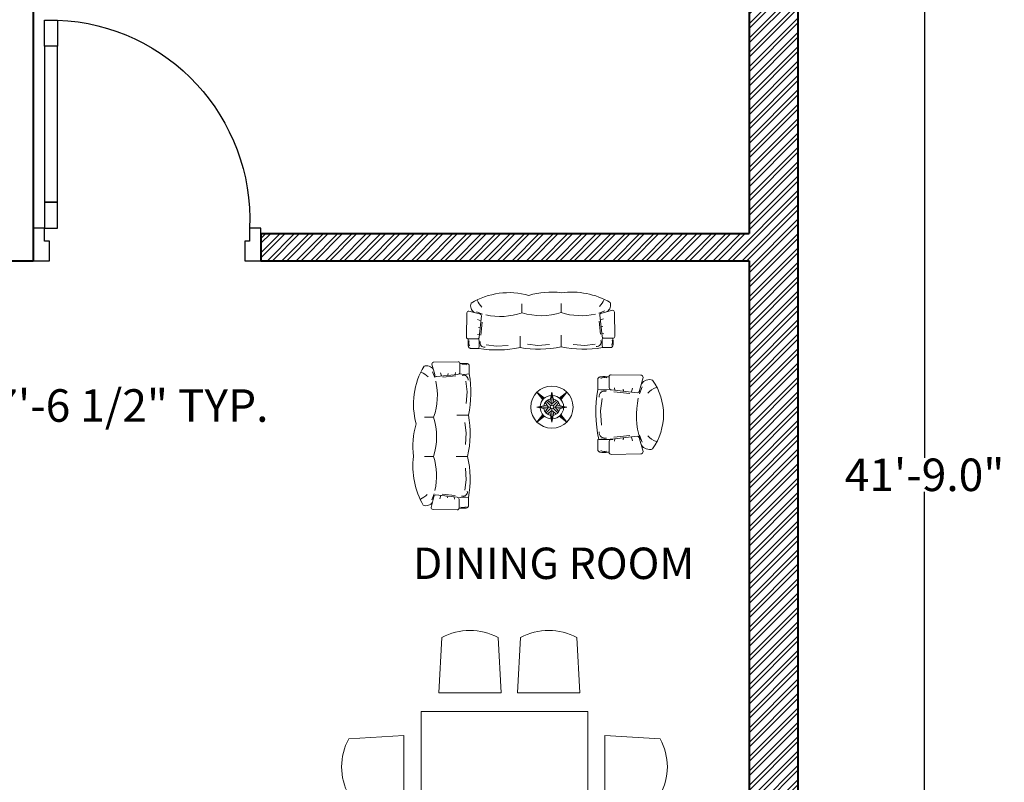
# Model space of a CAD drawing. Units: inches. Extents: x 528 to 2520, y -151 to 1354.
# Tile 21 of 41: x 1279 to 1461, y 1010 to 1151. Entities that reach past the tile are written whole.
import ezdxf

# ---------------------------------------------------------------- set-up
doc = ezdxf.new("R2010")
doc.units = ezdxf.units.IN
doc.header["$MEASUREMENT"] = 0
for name, color, linetype, lineweight in [('A-ANNO-DIMS', 2, 'Continuous', 18), ('A-AREA-IDEN', 7, 'Continuous', 18), ('A-Door', 150, 'Continuous', 25), ('A-FURN', 8, 'Continuous', 18), ('A-WALL-PATT', 6, 'Continuous', 13), ('walls', 7, 'Continuous', 40)]:
    doc.layers.add(name, color=color, linetype=linetype, lineweight=lineweight)
doc.layers.add('NT', color=1, linetype='Continuous')
doc.styles.get("Standard").update_dxf_attribs({"font": 'arial.ttf'})
doc.dimstyles.get("Standard").update_dxf_attribs({"dimtxt": 6, "dimasz": 2, "dimexe": 0.18, "dimexo": 0.0625, "dimgap": 0.09, "dimtad": 0, "dimtih": 1, "dimtoh": 1, "dimdec": 1, "dimzin": 0, "dimdsep": 46, "dimlunit": 3, "dimtxsty": 'Standard', "dimblk": 'ARCHTICK', "dimcen": 0.09, "dimadec": 0, "dimazin": 0, "dimtfac": 1, "dimtdec": 1, "dimtofl": 0, "dimtmove": 0, "dimatfit": 3, "dimfxl": 1, "dimtolj": 1, "dimtzin": 0, "dimarcsym": 0})

# ---------------------------------------------------------------- blocks, each defined once
blk = doc.blocks.new('A$C7DB75F4D')
at = {"layer": 'A-Door'}
for points in [[(625, 740), (625, 660), (665, 660), (665, 740)], [(625, 180), (625, 660), (665, 660), (665, 180)], [(625, 100), (625, 180), (665, 180), (665, 100)], [(35, 100), (35, 60), (50, 60), (50, 50), (50, 0), (0, 0), (0, 100)], [(665, 100), (700, 100), (700, 0), (650, 0), (650, 50), (650, 60), (665, 60)]]:
    blk.add_lwpolyline(points, close=True, dxfattribs=at)
at = {"layer": 'NT'}
blk.add_arc((650, 125), 615.5, 92.3278, 182.3278, dxfattribs=at)
blk = doc.blocks.new('table-20')
at = {"color": 0, "linetype": 'ByBlock'}
for p, q in [((-1.0518, 0.5326), (-1.074, 0.1341)), ((-0.6461, 0.5326), (-0.624, 0.1341)), ((-0.4837, 0.5326), (-0.5058, 0.1341)), ((-0.078, 0.5326), (-0.0558, 0.1341)), ((-0.624, 0.1341), (-1.074, 0.1341)), ((-0.0558, 0.1341), (-0.5058, 0.1341)), ((-1.2, 0), (0, 0)), ((-1.2, -0.8), (-1.2, 0)), ((0, -0.8), (0, 0)), ((-1.7227, -0.1971), (-1.3243, -0.175)), ((-1.3243, -0.625), (-1.3243, -0.175)), ((0.1243, -0.625), (0.1243, -0.175)), ((0.5227, -0.1971), (0.1243, -0.175)), ((-1.7227, -0.6029), (-1.3243, -0.625)), ((0.5227, -0.6029), (0.1243, -0.625)), ((-1.2, -0.8), (0, -0.8)), ((-0.624, -0.9341), (-1.074, -0.9341)), ((-1.0518, -1.3326), (-1.074, -0.9341)), ((-0.6461, -1.3326), (-0.624, -0.9341)), ((-0.4837, -1.3326), (-0.5058, -0.9341)), ((-0.0558, -0.9341), (-0.5058, -0.9341)), ((-0.078, -1.3326), (-0.0558, -0.9341))]:
    blk.add_line(p, q, dxfattribs=at)
for centre, start, end in [((-0.849, 0.1591), 61.48912, 118.51088), ((-0.2808, 0.1591), 61.48912, 118.51088), ((-1.3493, -0.4), 151.48912, 208.51088), ((0.1493, -0.4), 331.48912, 28.51088), ((-0.849, -0.9591), 241.48912, 298.51088), ((-0.2808, -0.9591), 241.48912, 298.51088)]:
    blk.add_arc(centre, 0.425, start, end, dxfattribs=at)
blk = doc.blocks.new('floor')
for p, q in [((-9.5, 11.5), (-18.9, 18.9)), ((-18.9, 18.9), (-10.6, 10.6)), ((-18.9, 18.9), (-11.6, 9.4)), ((0, 18.9), (-2.4, 6.1)), ((2.4, 6.1), (0, 18.9)), ((0, 18.9), (0, 2.1)), ((18.9, 18.9), (9.4, 11.5)), ((18.9, 18.9), (10.6, 10.6)), ((11.5, 9.4), (18.9, 18.9)), ((-6.1, 2.4), (-18.9, 0)), ((-18.9, 0), (-6.1, -2.4)), ((-18.9, 0), (-2.1, 0)), ((-8.7, 5.8), (-4.2, 0)), ((-7.4, 7.4), (-1.5, 1.5)), ((0, 4.2), (-5.8, 8.7)), ((5.8, 8.7), (0, 4.2)), ((7.4, 7.4), (1.5, 1.5)), ((2.1, 0), (18.9, 0)), ((4.2, 0), (8.7, 5.8)), ((18.9, 0), (6.1, 2.4)), ((6.1, -2.4), (18.9, 0)), ((-11.6, -9.5), (-18.9, -18.9)), ((-10.6, -10.6), (-18.9, -18.9)), ((-18.9, -18.9), (-9.5, -11.6)), ((-4.2, 0), (-8.7, -5.8)), ((-1.5, -1.5), (-7.4, -7.4)), ((-5.8, -8.7), (0, -4.2)), ((-2.4, -6.1), (0, -18.9)), ((0, -2.1), (0, -18.9)), ((0, -4.2), (5.8, -8.7)), ((0, -18.9), (2.4, -6.1)), ((1.5, -1.5), (7.4, -7.4)), ((8.7, -5.8), (4.2, 0)), ((9.4, -11.6), (18.9, -18.9)), ((10.6, -10.6), (18.9, -18.9)), ((18.9, -18.9), (11.5, -9.5))]:
    blk.add_line(p, q)
for radius in [26.7, 2.1]:
    blk.add_circle((0, 0), radius)
for radius, start, end in [(14.9, 92.8609, 177.1391), (14.9, 2.8609, 87.1391), (10.5, 98.7017, 171.2983), (10.5, 8.7017, 81.2983), (14.9, 182.8609, 267.1391), (10.5, 188.7017, 261.2983), (14.9, 272.8609, 357.1391), (10.5, 278.7017, 351.2983)]:
    blk.add_arc((0, 0), radius, start, end)
blk = doc.blocks.new('3-s')
for p, q in [((-3104.73, -915.45), (-3104.73, -919.55)), ((-3099.98, -914.27), (-3099.98, -918.75)), ((-3086.85, -913.54), (-3099.1, -913.37)), ((-3087.27, -919.9), (-3085.85, -914.54)), ((-3098.98, -919.75), (-3088.27, -920.9)), ((-3091.42, -921.25), (-3098, -920.58)), ((-3097.59, -919.77), (-3097.73, -918.83)), ((-3093.97, -920.17), (-3094.1, -919.37)), ((-3090.75, -920.58), (-3090.21, -918.96)), ((-3086.18, -918.42), (-3087.39, -921.38)), ((-3102.96, -923.27), (-3103.63, -928.52)), ((-3103.63, -928.52), (-3103.23, -934.44)), ((-3104.33, -940.39), (-3098.51, -940.39)), ((-3087.08, -940.39), (-3082.49, -940.39)), ((-3103.63, -952.27), (-3103.23, -946.35)), ((-3102.96, -957.52), (-3103.63, -952.27)), ((-3087.15, -960.23), (-3082.56, -960.23)), ((-3104.73, -961.23), (-3098.92, -961.23)), ((-3104.04, -973.11), (-3103.63, -967.19)), ((-3103.37, -978.36), (-3104.04, -973.11)), ((-3091.82, -980.37), (-3098.4, -981.05)), ((-3086.59, -983.2), (-3087.79, -980.24)), ((-3105.14, -986.18), (-3105.14, -982.07)), ((-3098, -981.85), (-3098.13, -982.8)), ((-3094.37, -981.45), (-3094.51, -982.26)), ((-3091.15, -981.05), (-3090.61, -982.66))]:
    blk.add_line(p, q)
for points in [[(-3099.98, -914.27), (-3100.65, -914.23), (-3101.21, -914.21), (-3101.68, -914.19), (-3102.07, -914.18), (-3102.4, -914.18), (-3102.68, -914.19), (-3102.91, -914.21), (-3103.11, -914.22), (-3103.29, -914.24), (-3103.46, -914.26), (-3103.62, -914.29), (-3103.76, -914.33), (-3103.89, -914.36), (-3104.01, -914.41), (-3104.12, -914.47), (-3104.23, -914.53), (-3104.33, -914.6), (-3104.43, -914.69), (-3104.51, -914.78), (-3104.58, -914.89), (-3104.65, -915.01), (-3104.69, -915.14), (-3104.72, -915.29), (-3104.73, -915.45)], [(-3100.39, -987.35), (-3101.05, -987.39), (-3101.61, -987.42), (-3102.08, -987.43), (-3102.48, -987.44), (-3102.81, -987.44), (-3103.08, -987.43), (-3103.31, -987.42), (-3103.51, -987.4), (-3103.7, -987.38), (-3103.87, -987.36), (-3104.02, -987.33), (-3104.16, -987.3), (-3104.29, -987.26), (-3104.41, -987.21), (-3104.53, -987.16), (-3104.63, -987.09), (-3104.73, -987.02), (-3104.83, -986.94), (-3104.91, -986.84), (-3104.99, -986.73), (-3105.05, -986.61), (-3105.1, -986.48), (-3105.13, -986.34), (-3105.14, -986.18)]]:
    blk.add_lwpolyline(points)
blk.add_lwpolyline([(-3087.67, -981.72), (-3086.25, -987.09, -0.414214), (-3087.25, -988.09), (-3099.51, -988.25, -0.464301), (-3100.39, -987.35), (-3100.39, -982.87, -0.414214), (-3099.39, -981.87), (-3088.67, -980.72, -0.414214)], format="xyb", close=True)
for centre, radius, start, end in [((-3101.91, -917.78), 3.27, 72.9324, 119.1125), ((-3099.16, -914.2), 0.826, 85.8896, 185.5116), ((-3086.85, -914.54), 1, 0, 90), ((-3083.18, -919.47), 4.05, 71.0879, 146.7483), ((-3117.09, -935.46), 40.42, 352.9967, 29.3731), ((-3051.57, -928.95), 53.99, 169.9808, 192.2408), ((-3102.44, -907.13), 12.63, 259.551, 282.5683), ((-3101.95, -922.43), 2.24, 70.9224, 187.7848), ((-3098.98, -918.75), 1, 180, 270), ((-3088.27, -919.9), 1, 270, 0), ((-3074.56, -931.19), 13.81, 115.1439, 132.7066), ((-3055.23, -930.36), 33.39, 167.467, 197.4804), ((-3051.57, -951.84), 53.99, 167.7592, 190.0192), ((-3055.23, -950.42), 33.39, 162.5196, 197.0763), ((-3117.09, -945.32), 40.42, 343.5213, 7.0033), ((-3055.63, -971.26), 33.39, 160.7021, 192.533), ((-3114.19, -966.81), 37.23, 329.0051, 15.6244), ((-3051.97, -972.68), 53.99, 167.7592, 190.0192), ((-3102.35, -979.2), 2.24, 172.2152, 289.0776), ((-3102.84, -994.5), 12.63, 77.4317, 100.449), ((-3083.58, -982.16), 4.05, 213.2517, 288.9121), ((-3074.97, -970.43), 13.81, 227.2934, 244.8561), ((-3102.31, -983.84), 3.27, 240.8875, 287.0676)]:
    blk.add_arc(centre, radius, start, end)
blk = doc.blocks.new('si-s')
for p, q in [((-3118, -943.94), (-3118, -948.05)), ((-3113.25, -942.77), (-3113.25, -947.25)), ((-3100.11, -942.03), (-3112.37, -941.87)), ((-3100.54, -948.4), (-3099.11, -943.03)), ((-3112.25, -948.25), (-3101.54, -949.4)), ((-3110.86, -948.27), (-3110.99, -947.32)), ((-3107.24, -948.67), (-3107.37, -947.86)), ((-3104.01, -949.07), (-3103.48, -947.46)), ((-3099.45, -946.92), (-3100.66, -949.88)), ((-3116.23, -951.76), (-3116.9, -957.01)), ((-3104.68, -949.75), (-3111.26, -949.07)), ((-3116.9, -957.01), (-3116.5, -962.93)), ((-3112.25, -968.73), (-3101.54, -967.58)), ((-3104.68, -967.23), (-3111.26, -967.9)), ((-3110.86, -968.71), (-3110.99, -969.65)), ((-3107.24, -968.31), (-3107.37, -969.11)), ((-3104.01, -967.9), (-3103.48, -969.52)), ((-3099.45, -970.06), (-3100.66, -967.1)), ((-3100.54, -968.58), (-3099.11, -973.94)), ((-3118, -973.03), (-3118, -968.93)), ((-3117.6, -968.89), (-3111.78, -968.89)), ((-3113.25, -974.21), (-3113.25, -969.73)), ((-3100.11, -974.94), (-3112.37, -975.11))]:
    blk.add_line(p, q)
for points in [[(-3113.25, -942.77), (-3113.92, -942.73), (-3114.48, -942.7), (-3114.95, -942.69), (-3115.34, -942.68), (-3115.67, -942.68), (-3115.94, -942.69), (-3116.18, -942.7), (-3116.38, -942.72), (-3116.56, -942.74), (-3116.73, -942.76), (-3116.88, -942.79), (-3117.03, -942.82), (-3117.16, -942.86), (-3117.28, -942.91), (-3117.39, -942.96), (-3117.5, -943.02), (-3117.6, -943.1), (-3117.69, -943.18), (-3117.78, -943.28), (-3117.85, -943.39), (-3117.91, -943.51), (-3117.96, -943.64), (-3117.99, -943.78), (-3118, -943.94)], [(-3113.25, -974.21), (-3113.92, -974.25), (-3114.48, -974.27), (-3114.95, -974.29), (-3115.34, -974.3), (-3115.67, -974.3), (-3115.94, -974.29), (-3116.18, -974.28), (-3116.38, -974.26), (-3116.56, -974.24), (-3116.73, -974.22), (-3116.88, -974.19), (-3117.03, -974.16), (-3117.16, -974.12), (-3117.28, -974.07), (-3117.39, -974.02), (-3117.5, -973.95), (-3117.6, -973.88), (-3117.69, -973.79), (-3117.78, -973.7), (-3117.85, -973.59), (-3117.91, -973.47), (-3117.96, -973.34), (-3117.99, -973.19), (-3118, -973.03)]]:
    blk.add_lwpolyline(points)
for centre, radius, start, end in [((-3115.18, -946.28), 3.27, 72.9324, 119.1125), ((-3112.43, -942.69), 0.826, 85.8896, 185.5116), ((-3100.11, -943.03), 1, 0, 90), ((-3096.45, -947.96), 4.05, 71.0879, 146.7483), ((-3115.55, -958.49), 24.96, 324.8902, 35.1098), ((-3064.84, -957.44), 53.99, 169.9808, 192.2408), ((-3115.71, -935.62), 12.63, 259.551, 282.5683), ((-3112.25, -947.25), 1, 180, 270), ((-3087.83, -959.69), 13.81, 115.1439, 132.7066), ((-3115.22, -950.92), 2.24, 70.9224, 187.7848), ((-3068.5, -958.86), 33.39, 167.467, 197.4804), ((-3101.54, -948.4), 1, 270, 0), ((-3115.71, -981.35), 12.63, 77.4317, 100.449), ((-3115.22, -966.05), 2.24, 172.2152, 289.0776), ((-3112.25, -969.73), 1, 90, 180), ((-3101.54, -968.58), 1, 0, 90), ((-3087.83, -957.29), 13.81, 227.2934, 244.8561), ((-3096.45, -969.01), 4.05, 213.2517, 288.9121), ((-3115.18, -970.7), 3.27, 240.8875, 287.0676), ((-3112.43, -974.29), 0.826, 174.4884, 274.1104), ((-3100.11, -973.94), 1, 270, 0)]:
    blk.add_arc(centre, radius, start, end)
blk = doc.blocks.new('_ArchTick')
at = {"color": 0, "linetype": 'ByBlock', "const_width": 0.15}
blk.add_lwpolyline([(-0.5, -0.5), (0.5, 0.5)], dxfattribs=at)
blk = doc.blocks.new('*D26')
at = {"layer": 'A-ANNO-DIMS', "color": 0, "lineweight": -2, "transparency": 16777216}
for p, q in [((1422.95, 1317.1), (1446.41, 1317.1)), ((1446.23, 1317.1), (1446.23, 1069.76)), ((1446.23, 816.1), (1446.23, 1063.45)), ((1422.95, 816.1), (1446.41, 816.1))]:
    blk.add_line(p, q, dxfattribs=at)
at = {"layer": 'Defpoints', "color": 0, "transparency": 16777216}
for p in [(1422.88, 1317.1), (1422.88, 816.1), (1446.23, 816.1)]:
    blk.add_point(p, dxfattribs=at)
at = {"layer": 'A-ANNO-DIMS', "color": 0, "lineweight": -2, "transparency": 16777216, "xscale": 2, "yscale": 2, "zscale": 2}
for p, rotation in [((1446.23, 1317.1), 90), ((1446.23, 816.1), 270)]:
    blk.add_blockref('_ArchTick', p, dxfattribs=dict(at, rotation=rotation))
at = {"layer": 'A-ANNO-DIMS', "color": 0, "transparency": 16777216, "insert": (1446.23, 1066.6), "char_height": 6, "attachment_point": 5}
blk.add_mtext('\\A1;41\'-9.0"', dxfattribs=at)
blk = doc.blocks.new('*D58')
at = {"layer": 'A-ANNO-DIMS', "color": 0, "lineweight": -2, "transparency": 16777216}
for p, q in [((1132.88, 1092.9), (1132.88, 1079.21)), ((1223.4, 1092.9), (1223.4, 1079.21)), ((1132.88, 1079.39), (1223.4, 1079.39)), ((1223.4, 1079.39), (1225.4, 1079.39))]:
    blk.add_line(p, q, dxfattribs=at)
at = {"layer": 'Defpoints', "color": 0, "transparency": 16777216}
for p in [(1132.88, 1092.96), (1223.4, 1092.96), (1223.4, 1079.39)]:
    blk.add_point(p, dxfattribs=at)
at = {"layer": 'A-ANNO-DIMS', "color": 0, "lineweight": -2, "transparency": 16777216, "xscale": 2, "yscale": 2, "zscale": 2, "rotation": 180}
blk.add_blockref('_ArchTick', (1132.88, 1079.39), dxfattribs=at)
at = {"layer": 'A-ANNO-DIMS', "color": 0, "lineweight": -2, "transparency": 16777216, "xscale": 2, "yscale": 2, "zscale": 2}
blk.add_blockref('_ArchTick', (1223.4, 1079.39), dxfattribs=at)
at = {"layer": 'A-ANNO-DIMS', "color": 0, "transparency": 16777216, "insert": (1276.74, 1079.39), "char_height": 6, "attachment_point": 5}
blk.add_mtext('\\A1;WARDROBE 7\'-6 1/2" TYP.', dxfattribs=at)

msp = doc.modelspace()

# ---------------------------------------------------------------- hatches: boundary and pattern name
at = {"layer": 'A-WALL-PATT'}
h = msp.add_hatch(dxfattribs=at)
h.set_pattern_fill('ANSI32', color=256, scale=5)
h.set_pattern_definition([(45, (537.1868, 0), (-1.3258252, 1.3258252), []), (45, (538.0707, 0), (-1.3258252, 1.3258252), [])])
h.paths.add_polyline_path([(1132.88, 1163.86), (1123.88, 1163.86), (1123.88, 969.1), (1135.43, 969.1), (1140.43, 969.1), (1140.43, 974.1), (1132.88, 974.1), (1132.88, 1082.1), (1228.88, 1082.1), (1228.88, 1087.1), (1228.88, 1106.1), (1234.88, 1106.1), (1234.88, 1111.1), (1223.88, 1111.1), (1223.88, 1087.1), (1132.88, 1087.1)])
h.paths.add_polyline_path([(1225.89, 974.1), (1188.43, 974.1), (1188.43, 969.1), (1225.89, 969.1)])
h.paths.add_polyline_path([(1422.88, 1171.37), (1413.88, 1171.37), (1413.88, 1111.1), (1323.88, 1111.1), (1323.88, 1106.1), (1413.88, 1106.1), (1413.88, 974.1), (1323.88, 974.1), (1323.88, 969.1), (1413.88, 969.1), (1413.88, 825.1), (1371.88, 825.1), (1371.88, 816.1), (1422.88, 816.1)])
h.paths.add_polyline_path([(1422.88, 1317.1), (1413.84, 1317.1), (1413.84, 1308.1), (1413.88, 1308.1), (1413.88, 1248.1), (1359.88, 1248.1), (1359.88, 1243.1), (1413.88, 1243.1), (1413.88, 1219.37), (1422.88, 1219.37)])
h.paths.add_polyline_path([(1389.84, 1317.1), (1324.88, 1317.1), (1324.88, 1248.1), (1321.45, 1248.1), (1321.45, 1243.1), (1329.88, 1243.1), (1329.88, 1249.1), (1329.88, 1308.1), (1389.84, 1308.1)])
h.paths.add_polyline_path([(1221.88, 1317.1), (1156.88, 1317.1), (1156.88, 1308.1), (1216.88, 1308.1), (1216.88, 1248.1), (1216.88, 1243.1), (1221.88, 1243.1), (1221.88, 1248.25)])
h.paths.add_polyline_path([(1132.88, 1308.1), (1132.88, 1317.1), (1123.88, 1317.1), (1123.88, 1211.86), (1132.88, 1211.86), (1132.88, 1243.1), (1186.88, 1243.1), (1186.88, 1248.1), (1132.88, 1248.1)])
h.paths.add_polyline_path([(1281.88, 969.1), (1281.88, 974.1), (1261.89, 974.1), (1261.89, 969.1), (1276.88, 969.1), (1276.88, 874.29), (1281.88, 874.29)])
h.paths.add_polyline_path([(1276.88, 969.1), (1264.88, 969.1), (1264.88, 965.12), (1267.92, 965.12), (1267.92, 961.68), (1271.62, 961.68), (1271.62, 957.24), (1276.88, 957.24)], flags=17)
h.paths.add_polyline_path([(1323.88, 825.1), (1281.88, 825.1), (1281.88, 832.29), (1276.88, 832.29), (1276.88, 816.1), (1323.88, 816.1)])

# ---------------------------------------------------------------- linework, layer by layer
at = {"layer": 'walls'}
for p, q in [((1422.88, 1317.1), (1422.88, 816.1)), ((1281.88, 1243.1), (1281.88, 1111.1)), ((1413.88, 1243.1), (1413.88, 1111.1)), ((1281.88, 1111.1), (1281.88, 1106.1)), ((1323.88, 1111.1), (1413.88, 1111.1)), ((1323.88, 1111.1), (1323.88, 1106.1)), ((1276.88, 1106.1), (1281.88, 1106.1)), ((1323.88, 1106.1), (1413.88, 1106.1)), ((1413.88, 1106.1), (1413.88, 974.1))]:
    msp.add_line(p, q, dxfattribs=at)

# ---------------------------------------------------------------- block references
at = {"layer": 'A-Door', "xscale": -0.0600000000000059, "yscale": 0.0600000000000059, "zscale": 0.0600000000000059}
msp.add_blockref('A$C7DB75F4D', (1323.88, 1106.1), dxfattribs=at)
at = {"layer": 'A-FURN'}
for p, xscale, yscale, zscale, rotation in [((1722.32, 2222.75), -0.3648213827119744, 0.3648213827119744, 0.3648213827119362, 270), ((229.46, 726.93), 0.3648213827118212, 0.3648213827118212, 0.3648213827118212, 180)]:
    msp.add_blockref('3-s', p, dxfattribs=dict(at, xscale=xscale, yscale=yscale, zscale=zscale, rotation=rotation))
for name, p, xscale, yscale, zscale in [('si-s', (2764.93, 1501.62), 0.4422535540881025, 0.4422535540881025, 0.4422535540881025), ('floor', (1377.52, 1079.09, -157.77), 0.1459285530847694, 0.1459285530847694, 0.1459285530847694), ('table-20', (1384.12, 1022.96), 25.57841077690889, 25.57841077690889, 25.57841077690889)]:
    msp.add_blockref(name, p, dxfattribs=dict(at, xscale=xscale, yscale=yscale, zscale=zscale))

# ---------------------------------------------------------------- texts
at = {"layer": 'A-AREA-IDEN'}
msp.add_text('DINING ROOM', height=5.7926, dxfattribs=at).set_placement((1351.89, 1047.38))

# ---------------------------------------------------------------- dimensions: what is measured, and where the dimension line sits
at = {"layer": 'A-ANNO-DIMS'}
dim = msp.add_linear_dim(base=(1446.23, 816.1), p1=(1422.88, 1317.1), p2=(1422.88, 816.1), angle=90, dimstyle='Standard', override={"dimclrd": 0, "dimclre": 0, "dimclrt": 0}, dxfattribs=at)
dim.commit()
dim.dimension.update_dxf_attribs({"geometry": '*D26', "text_midpoint": (1446.23, 1066.6)})
dim = msp.add_linear_dim(base=(1223.4, 1079.39), p1=(1132.88, 1092.96), p2=(1223.4, 1092.96), text='WARDROBE <> TYP.', dimstyle='Standard', override={"dimdec": 1, "dimlfac": 1, "dimrnd": 0, "dimzin": 1, "dimdsep": 46, "dimlunit": 4, "dimfrac": 2}, dxfattribs=at)
dim.commit()
dim.dimension.update_dxf_attribs({"geometry": '*D58', "text_midpoint": (1276.74, 1079.39)})

doc.saveas('drawing.dxf')
